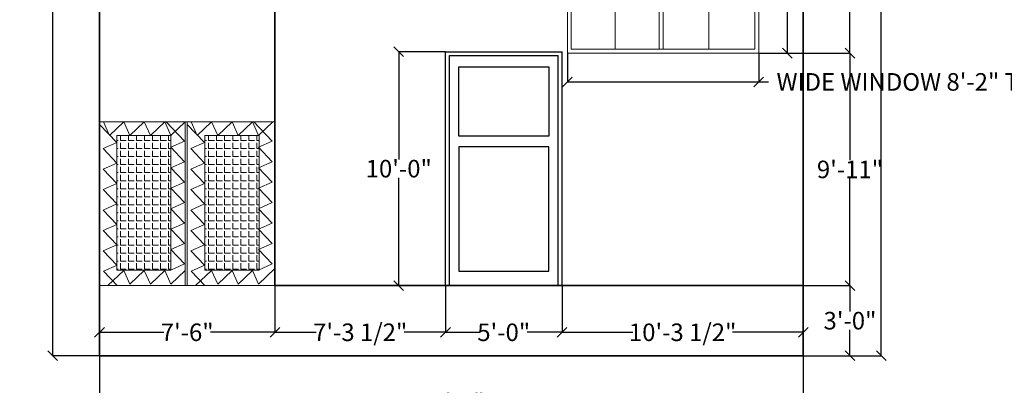
# Model space of a CAD drawing. Units: inches. Extents: x -19 to 1000, y -122 to 1144.
# Tile 6 of 8: x -19 to 486, y 313 to 501. Entities that reach past the tile are written whole.
import ezdxf

# ---------------------------------------------------------------- set-up
doc = ezdxf.new("R2010")
doc.units = ezdxf.units.IN
doc.header["$MEASUREMENT"] = 0
for name, color, linetype, lineweight in [('A-ANNO-DIMS', 191, 'Continuous', 18), ('A-ELEV', 4, 'Continuous', 35), ('A-ELEV-DOOR', 2, 'Continuous', 25), ('A-ELEV-GATE', 4, 'Continuous', 18), ('A-ELEV-GLAZ', 3, 'Continuous', 18), ('A-ELEV-PATT', 8, 'Continuous', 13)]:
    doc.layers.add(name, color=color, linetype=linetype, lineweight=lineweight)
doc.styles.get("Standard").update_dxf_attribs({"font": 'arial.ttf'})
doc.dimstyles.get("Standard").update_dxf_attribs({"dimtxt": 9, "dimasz": 5, "dimexe": 0.18, "dimexo": 0.0625, "dimgap": 0.09, "dimtad": 0, "dimtih": 1, "dimtoh": 1, "dimdec": 0, "dimzin": 0, "dimdsep": 46, "dimlunit": 3, "dimtxsty": 'Standard', "dimblk": 'OBLIQUE', "dimcen": 0.09, "dimadec": 0, "dimazin": 0, "dimtfac": 1, "dimtdec": 0, "dimtofl": 0, "dimtmove": 0, "dimatfit": 3, "dimfxl": 1, "dimtolj": 1, "dimtzin": 0, "dimarcsym": 0})

# ---------------------------------------------------------------- blocks, each defined once
blk = doc.blocks.new('_Oblique')
at = {"color": 0, "linetype": 'ByBlock', "lineweight": -2}
blk.add_line((-0.5, -0.5), (0.5, 0.5), dxfattribs=at)
blk = doc.blocks.new('*D9')
at = {"layer": 'A-ANNO-DIMS', "color": 0, "lineweight": -2, "transparency": 16777216}
for p, q in [((382.7, 727.13), (422.85, 727.13)), ((422.67, 727.13), (422.67, 532.32)), ((422.67, 328.13), (422.67, 522.95)), ((382.7, 328.13), (422.85, 328.13))]:
    blk.add_line(p, q, dxfattribs=at)
at = {"layer": 'Defpoints', "color": 0, "transparency": 16777216}
for p in [(382.64, 727.13), (422.67, 727.13), (382.64, 328.13)]:
    blk.add_point(p, dxfattribs=at)
at = {"layer": 'A-ANNO-DIMS', "color": 0, "lineweight": -2, "transparency": 16777216, "xscale": 5, "yscale": 5, "zscale": 5}
for p, rotation in [((422.67, 727.13), 90), ((422.67, 328.13), 270)]:
    blk.add_blockref('_Oblique', p, dxfattribs=dict(at, rotation=rotation))
at = {"layer": 'A-ANNO-DIMS', "color": 0, "transparency": 16777216, "insert": (422.67, 527.63), "char_height": 9, "attachment_point": 5}
blk.add_mtext('\\A1;33\'-3"', dxfattribs=at)
blk = doc.blocks.new('WINDOW-ELEV-WIDE')
for p, q in [((47.06, 49.36), (47.06, 64.32)), ((49.06, 49.36), (49.06, 64.32)), ((2, 49.36), (47.06, 49.36)), ((2, 47.36), (47.06, 47.36)), ((24.53, 47.36), (24.53, 2)), ((47.06, 2), (47.06, 47.36)), ((49.06, 49.36), (96.11, 49.36)), ((49.06, 2), (49.06, 47.36)), ((49.06, 47.36), (96.11, 47.36)), ((72.58, 47.36), (72.58, 2))]:
    blk.add_line(p, q)
for points in [[(98.11, 0), (0, 0), (0, 66.32), (98.11, 66.32)], [(96.11, 2), (2, 2), (2, 64.32), (96.11, 64.32)]]:
    blk.add_lwpolyline(points, close=True)
blk = doc.blocks.new('*D73')
at = {"layer": 'A-ANNO-DIMS', "color": 0, "lineweight": -2, "transparency": 16777216}
for p, q in [((261.67, 483.28), (261.67, 468.45)), ((359.78, 483.28), (359.78, 468.45)), ((261.67, 468.63), (359.78, 468.63)), ((359.78, 468.63), (364.78, 468.63))]:
    blk.add_line(p, q, dxfattribs=at)
at = {"layer": 'Defpoints', "color": 0, "transparency": 16777216}
for p in [(261.67, 483.35), (359.78, 483.35), (359.78, 468.63)]:
    blk.add_point(p, dxfattribs=at)
at = {"layer": 'A-ANNO-DIMS', "color": 0, "lineweight": -2, "transparency": 16777216, "xscale": 5, "yscale": 5, "zscale": 5, "rotation": 180}
blk.add_blockref('_Oblique', (261.67, 468.63), dxfattribs=at)
at = {"layer": 'A-ANNO-DIMS', "color": 0, "lineweight": -2, "transparency": 16777216, "xscale": 5, "yscale": 5, "zscale": 5}
blk.add_blockref('_Oblique', (359.78, 468.63), dxfattribs=at)
at = {"layer": 'A-ANNO-DIMS', "color": 0, "transparency": 16777216, "insert": (439.97, 468.63), "char_height": 9, "attachment_point": 5}
blk.add_mtext('\\A1;WIDE WINDOW 8\'-2" TYP.', dxfattribs=at)
blk = doc.blocks.new('*D74')
at = {"layer": 'A-ANNO-DIMS', "color": 0, "lineweight": -2, "transparency": 16777216}
for p, q in [((359.84, 549.66), (374.68, 549.66)), ((374.5, 549.66), (374.5, 521.25)), ((374.5, 483.35), (374.5, 511.76)), ((359.84, 483.35), (374.68, 483.35))]:
    blk.add_line(p, q, dxfattribs=at)
at = {"layer": 'Defpoints', "color": 0, "transparency": 16777216}
for p in [(359.78, 549.66), (374.5, 549.66), (359.78, 483.35)]:
    blk.add_point(p, dxfattribs=at)
at = {"layer": 'A-ANNO-DIMS', "color": 0, "lineweight": -2, "transparency": 16777216, "xscale": 5, "yscale": 5, "zscale": 5}
for p, rotation in [((374.5, 549.66), 90), ((374.5, 483.35), 270)]:
    blk.add_blockref('_Oblique', p, dxfattribs=dict(at, rotation=rotation))
at = {"layer": 'A-ANNO-DIMS', "color": 0, "transparency": 16777216, "insert": (374.5, 516.51), "char_height": 9, "attachment_point": 5}
blk.add_mtext('\\A1;5\'-6 1/2" TYP.', dxfattribs=at)
blk = doc.blocks.new('*D78')
at = {"layer": 'A-ANNO-DIMS', "color": 0, "lineweight": -2, "transparency": 16777216}
for p, q in [((61.2, 524.21), (61.2, 509.56)), ((83.4, 524.21), (83.4, 509.56)), ((61.2, 509.74), (83.4, 509.74)), ((83.4, 509.74), (88.4, 509.74))]:
    blk.add_line(p, q, dxfattribs=at)
at = {"layer": 'Defpoints', "color": 0, "transparency": 16777216}
for p in [(61.2, 524.27), (83.4, 524.27), (83.4, 509.74)]:
    blk.add_point(p, dxfattribs=at)
at = {"layer": 'A-ANNO-DIMS', "color": 0, "lineweight": -2, "transparency": 16777216, "xscale": 5, "yscale": 5, "zscale": 5, "rotation": 180}
blk.add_blockref('_Oblique', (61.2, 509.74), dxfattribs=at)
at = {"layer": 'A-ANNO-DIMS', "color": 0, "lineweight": -2, "transparency": 16777216, "xscale": 5, "yscale": 5, "zscale": 5}
blk.add_blockref('_Oblique', (83.4, 509.74), dxfattribs=at)
at = {"layer": 'A-ANNO-DIMS', "color": 0, "transparency": 16777216, "insert": (118.99, 509.74), "char_height": 9, "attachment_point": 5}
blk.add_mtext('\\A1;1\'-10" TYP.', dxfattribs=at)
blk = doc.blocks.new('*D111')
at = {"layer": 'A-ANNO-DIMS', "color": 0, "lineweight": -2, "transparency": 16777216}
for p, q in [((21.64, 328.07), (21.64, 304)), ((382.64, 328.07), (382.64, 304)), ((21.64, 304.18), (186.6, 304.18)), ((382.64, 304.18), (217.69, 304.18))]:
    blk.add_line(p, q, dxfattribs=at)
at = {"layer": 'Defpoints', "color": 0, "transparency": 16777216}
for p in [(21.64, 328.13), (382.64, 328.13), (21.64, 304.18)]:
    blk.add_point(p, dxfattribs=at)
at = {"layer": 'A-ANNO-DIMS', "color": 0, "lineweight": -2, "transparency": 16777216, "xscale": 5, "yscale": 5, "zscale": 5, "rotation": 180}
blk.add_blockref('_Oblique', (21.64, 304.18), dxfattribs=at)
at = {"layer": 'A-ANNO-DIMS', "color": 0, "lineweight": -2, "transparency": 16777216, "xscale": 5, "yscale": 5, "zscale": 5}
blk.add_blockref('_Oblique', (382.64, 304.18), dxfattribs=at)
at = {"layer": 'A-ANNO-DIMS', "color": 0, "transparency": 16777216, "insert": (202.14, 304.18), "char_height": 9, "attachment_point": 5}
blk.add_mtext('\\A1;30\'-1"', dxfattribs=at)
blk = doc.blocks.new('*D112')
at = {"layer": 'A-ANNO-DIMS', "color": 0, "lineweight": -2, "transparency": 16777216}
for p, q in [((21.58, 797.3), (-2.49, 797.3)), ((-2.31, 797.3), (-2.31, 567.4)), ((-2.31, 328.13), (-2.31, 558.03)), ((21.58, 328.13), (-2.49, 328.13))]:
    blk.add_line(p, q, dxfattribs=at)
at = {"layer": 'Defpoints', "color": 0, "transparency": 16777216}
for p in [(-2.31, 797.3), (21.64, 797.3), (21.64, 328.13)]:
    blk.add_point(p, dxfattribs=at)
at = {"layer": 'A-ANNO-DIMS', "color": 0, "lineweight": -2, "transparency": 16777216, "xscale": 5, "yscale": 5, "zscale": 5}
for p, rotation in [((-2.31, 797.3), 90), ((-2.31, 328.13), 270)]:
    blk.add_blockref('_Oblique', p, dxfattribs=dict(at, rotation=rotation))
at = {"layer": 'A-ANNO-DIMS', "color": 0, "transparency": 16777216, "insert": (-2.31, 562.72), "char_height": 9, "attachment_point": 5}
blk.add_mtext('\\A1;39\'-1"', dxfattribs=at)
blk = doc.blocks.new('*D113')
at = {"layer": 'A-ANNO-DIMS', "color": 0, "lineweight": -2, "transparency": 16777216}
for p, q in [((21.64, 364.07), (21.64, 340)), ((111.64, 364.07), (111.64, 340)), ((21.64, 340.18), (54.63, 340.18)), ((111.64, 340.18), (78.66, 340.18))]:
    blk.add_line(p, q, dxfattribs=at)
at = {"layer": 'Defpoints', "color": 0, "transparency": 16777216}
for p in [(21.64, 364.13), (111.64, 364.13), (21.64, 340.18)]:
    blk.add_point(p, dxfattribs=at)
at = {"layer": 'A-ANNO-DIMS', "color": 0, "lineweight": -2, "transparency": 16777216, "xscale": 5, "yscale": 5, "zscale": 5, "rotation": 180}
blk.add_blockref('_Oblique', (21.64, 340.18), dxfattribs=at)
at = {"layer": 'A-ANNO-DIMS', "color": 0, "lineweight": -2, "transparency": 16777216, "xscale": 5, "yscale": 5, "zscale": 5}
blk.add_blockref('_Oblique', (111.64, 340.18), dxfattribs=at)
at = {"layer": 'A-ANNO-DIMS', "color": 0, "transparency": 16777216, "insert": (66.64, 340.18), "char_height": 9, "attachment_point": 5}
blk.add_mtext('\\A1;7\'-6"', dxfattribs=at)
blk = doc.blocks.new('*D114')
at = {"layer": 'A-ANNO-DIMS', "color": 0, "lineweight": -2, "transparency": 16777216}
for p, q in [((111.64, 364.07), (111.64, 340)), ((199.11, 364.07), (199.11, 340)), ((111.64, 340.18), (132.87, 340.18)), ((199.11, 340.18), (177.88, 340.18))]:
    blk.add_line(p, q, dxfattribs=at)
at = {"layer": 'Defpoints', "color": 0, "transparency": 16777216}
for p in [(111.64, 364.13), (199.11, 364.13), (111.64, 340.18)]:
    blk.add_point(p, dxfattribs=at)
at = {"layer": 'A-ANNO-DIMS', "color": 0, "lineweight": -2, "transparency": 16777216, "xscale": 5, "yscale": 5, "zscale": 5, "rotation": 180.0000000000001}
blk.add_blockref('_Oblique', (111.64, 340.18), dxfattribs=at)
at = {"layer": 'A-ANNO-DIMS', "color": 0, "lineweight": -2, "transparency": 16777216, "xscale": 5, "yscale": 5, "zscale": 5}
blk.add_blockref('_Oblique', (199.11, 340.18), dxfattribs=at)
at = {"layer": 'A-ANNO-DIMS', "color": 0, "transparency": 16777216, "insert": (155.38, 340.18), "char_height": 9, "attachment_point": 5}
blk.add_mtext('\\A1;7\'-3 1/2"', dxfattribs=at)
blk = doc.blocks.new('*D115')
at = {"layer": 'A-ANNO-DIMS', "color": 0, "lineweight": -2, "transparency": 16777216}
for p, q in [((199.11, 364.07), (199.11, 340)), ((258.9, 364.07), (258.9, 340)), ((199.11, 340.18), (216.95, 340.18)), ((258.9, 340.18), (241.06, 340.18))]:
    blk.add_line(p, q, dxfattribs=at)
at = {"layer": 'Defpoints', "color": 0, "transparency": 16777216}
for p in [(199.11, 364.13), (258.9, 364.13), (199.11, 340.18)]:
    blk.add_point(p, dxfattribs=at)
at = {"layer": 'A-ANNO-DIMS', "color": 0, "lineweight": -2, "transparency": 16777216, "xscale": 5, "yscale": 5, "zscale": 5, "rotation": 180}
blk.add_blockref('_Oblique', (199.11, 340.18), dxfattribs=at)
at = {"layer": 'A-ANNO-DIMS', "color": 0, "lineweight": -2, "transparency": 16777216, "xscale": 5, "yscale": 5, "zscale": 5}
blk.add_blockref('_Oblique', (258.9, 340.18), dxfattribs=at)
at = {"layer": 'A-ANNO-DIMS', "color": 0, "transparency": 16777216, "insert": (229, 340.18), "char_height": 9, "attachment_point": 5}
blk.add_mtext('\\A1;5\'-0"', dxfattribs=at)
blk = doc.blocks.new('*D116')
at = {"layer": 'A-ANNO-DIMS', "color": 0, "lineweight": -2, "transparency": 16777216}
for p, q in [((258.9, 364.07), (258.9, 340)), ((382.64, 364.07), (382.64, 340)), ((258.9, 340.18), (295.16, 340.18)), ((382.64, 340.18), (346.38, 340.18))]:
    blk.add_line(p, q, dxfattribs=at)
at = {"layer": 'Defpoints', "color": 0, "transparency": 16777216}
for p in [(258.9, 364.13), (382.64, 364.13), (258.9, 340.18)]:
    blk.add_point(p, dxfattribs=at)
at = {"layer": 'A-ANNO-DIMS', "color": 0, "lineweight": -2, "transparency": 16777216, "xscale": 5, "yscale": 5, "zscale": 5}
for p, rotation in [((258.9, 340.18), 179.9999999999999), ((382.64, 340.18), 359.9999999999999)]:
    blk.add_blockref('_Oblique', p, dxfattribs=dict(at, rotation=rotation))
at = {"layer": 'A-ANNO-DIMS', "color": 0, "transparency": 16777216, "insert": (320.77, 340.18), "char_height": 9, "attachment_point": 5}
blk.add_mtext('\\A1;10\'-3 1/2"', dxfattribs=at)
blk = doc.blocks.new('*D117')
at = {"layer": 'A-ANNO-DIMS', "color": 0, "lineweight": -2, "transparency": 16777216}
for p, q in [((382.7, 364.13), (406.77, 364.13)), ((406.59, 364.13), (406.59, 350.82)), ((406.59, 328.13), (406.59, 341.45)), ((382.7, 328.13), (406.77, 328.13))]:
    blk.add_line(p, q, dxfattribs=at)
at = {"layer": 'Defpoints', "color": 0, "transparency": 16777216}
for p in [(382.64, 364.13), (406.59, 364.13), (382.64, 328.13)]:
    blk.add_point(p, dxfattribs=at)
at = {"layer": 'A-ANNO-DIMS', "color": 0, "lineweight": -2, "transparency": 16777216, "xscale": 5, "yscale": 5, "zscale": 5}
for p, rotation in [((406.59, 364.13), 90), ((406.59, 328.13), 270)]:
    blk.add_blockref('_Oblique', p, dxfattribs=dict(at, rotation=rotation))
at = {"layer": 'A-ANNO-DIMS', "color": 0, "transparency": 16777216, "insert": (406.59, 346.13), "char_height": 9, "attachment_point": 5}
blk.add_mtext('\\A1;3\'-0"', dxfattribs=at)
blk = doc.blocks.new('*D118')
at = {"layer": 'A-ANNO-DIMS', "color": 0, "lineweight": -2, "transparency": 16777216}
for p, q in [((199.05, 484.13), (174.98, 484.13)), ((175.16, 484.13), (175.16, 428.82)), ((175.16, 364.13), (175.16, 419.45)), ((199.05, 364.13), (174.98, 364.13))]:
    blk.add_line(p, q, dxfattribs=at)
at = {"layer": 'Defpoints', "color": 0, "transparency": 16777216}
for p in [(175.16, 484.13), (199.11, 484.13), (199.11, 364.13)]:
    blk.add_point(p, dxfattribs=at)
at = {"layer": 'A-ANNO-DIMS', "color": 0, "lineweight": -2, "transparency": 16777216, "xscale": 5, "yscale": 5, "zscale": 5}
for p, rotation in [((175.16, 484.13), 90), ((175.16, 364.13), 270)]:
    blk.add_blockref('_Oblique', p, dxfattribs=dict(at, rotation=rotation))
at = {"layer": 'A-ANNO-DIMS', "color": 0, "transparency": 16777216, "insert": (175.16, 424.13), "char_height": 9, "attachment_point": 5}
blk.add_mtext('\\A1;10\'-0"', dxfattribs=at)
blk = doc.blocks.new('*D121')
at = {"layer": 'A-ANNO-DIMS', "color": 0, "lineweight": -2, "transparency": 16777216}
for p, q in [((359.84, 483.35), (406.77, 483.35)), ((406.59, 483.35), (406.59, 428.43)), ((406.59, 364.13), (406.59, 419.06)), ((382.7, 364.13), (406.77, 364.13))]:
    blk.add_line(p, q, dxfattribs=at)
at = {"layer": 'Defpoints', "color": 0, "transparency": 16777216}
for p in [(359.78, 483.35), (406.59, 483.35), (382.64, 364.13)]:
    blk.add_point(p, dxfattribs=at)
at = {"layer": 'A-ANNO-DIMS', "color": 0, "lineweight": -2, "transparency": 16777216, "xscale": 5, "yscale": 5, "zscale": 5}
for p, rotation in [((406.59, 483.35), 90), ((406.59, 364.13), 270)]:
    blk.add_blockref('_Oblique', p, dxfattribs=dict(at, rotation=rotation))
at = {"layer": 'A-ANNO-DIMS', "color": 0, "transparency": 16777216, "insert": (406.59, 423.74), "char_height": 9, "attachment_point": 5}
blk.add_mtext('\\A1;9\'-11"', dxfattribs=at)
blk = doc.blocks.new('*D122')
at = {"layer": 'A-ANNO-DIMS', "color": 0, "lineweight": -2, "transparency": 16777216}
for p, q in [((382.7, 613.85), (406.77, 613.85)), ((406.59, 613.85), (406.59, 553.34)), ((406.59, 483.35), (406.59, 543.86)), ((359.84, 483.35), (406.77, 483.35))]:
    blk.add_line(p, q, dxfattribs=at)
at = {"layer": 'Defpoints', "color": 0, "transparency": 16777216}
for p in [(382.64, 613.85), (406.59, 613.85), (359.78, 483.35)]:
    blk.add_point(p, dxfattribs=at)
at = {"layer": 'A-ANNO-DIMS', "color": 0, "lineweight": -2, "transparency": 16777216, "xscale": 5, "yscale": 5, "zscale": 5}
for p, rotation in [((406.59, 613.85), 90), ((406.59, 483.35), 270)]:
    blk.add_blockref('_Oblique', p, dxfattribs=dict(at, rotation=rotation))
at = {"layer": 'A-ANNO-DIMS', "color": 0, "transparency": 16777216, "insert": (406.59, 548.6), "char_height": 9, "attachment_point": 5}
blk.add_mtext('\\A1;10\'-10 1/2"', dxfattribs=at)

msp = doc.modelspace()

# ---------------------------------------------------------------- hatches: boundary and pattern name
at = {"layer": 'A-ELEV-PATT'}
h = msp.add_hatch(dxfattribs=at)
h.set_pattern_fill('ANGLE', color=256, scale=15)
h.set_pattern_definition([(0, (-437.899, -266.802), (0, 4.125), [3, -1.125]), (90, (-437.899, -266.802), (-4.125, 3e-16), [3, -1.125])])
h.paths.add_polyline_path([(58.27, 441.14), (30.51, 441.14), (30.51, 372.1), (58.27, 372.1)])
h = msp.add_hatch(dxfattribs=at)
h.set_pattern_fill('ANGLE', color=256, scale=15)
h.set_pattern_definition([(0, (-392.659, -266.802), (0, 4.125), [3, -1.125]), (90, (-392.659, -266.802), (-4.125, 3e-16), [3, -1.125])])
h.paths.add_polyline_path([(103.51, 441.14), (75.75, 441.14), (75.75, 372.1), (103.51, 372.1)])

# ---------------------------------------------------------------- linework, layer by layer
at = {"layer": 'A-ELEV'}
for p, q in [((21.64, 328.13), (21.64, 727.13)), ((111.64, 364.13), (111.64, 727.13)), ((382.64, 328.13), (382.64, 727.13)), ((382.64, 328.13), (382.64, 727.13)), ((382.64, 364.13), (111.64, 364.13)), ((382.64, 328.13), (21.64, 328.13))]:
    msp.add_line(p, q, dxfattribs=at)
at = {"layer": 'A-ELEV-DOOR'}
for p, q in [((199.11, 364.13), (199.11, 484.13)), ((199.11, 484.13), (258.9, 484.13)), ((201.11, 482.13), (256.9, 482.13)), ((201.11, 364.13), (201.11, 482.13)), ((256.9, 364.13), (256.9, 482.13)), ((258.9, 364.13), (258.9, 484.13))]:
    msp.add_line(p, q, dxfattribs=at)
for points in [[(252.13, 440.81), (206.02, 440.81), (206.02, 476.32), (252.13, 476.32)], [(252.13, 435.3), (206.02, 435.3), (206.02, 371.57), (252.13, 371.57)]]:
    msp.add_lwpolyline(points, close=True, dxfattribs=at)
at = {"layer": 'A-ELEV-GATE'}
for p, q in [((111.64, 448.13), (21.64, 448.13)), ((21.64, 446.86), (30.51, 437.5)), ((26.78, 441.14), (23.66, 448.13)), ((26.78, 441.14), (34.15, 448.13)), ((37.28, 441.14), (34.15, 448.13)), ((37.28, 441.14), (44.65, 448.13)), ((47.77, 441.14), (44.65, 448.13)), ((47.77, 441.14), (55.15, 448.13)), ((58.27, 441.14), (55.15, 448.13)), ((65.26, 438.2), (55.84, 448.13)), ((58.27, 441.14), (65.64, 448.13)), ((65.64, 364.13), (65.64, 448.13)), ((66.64, 364.13), (66.64, 448.13)), ((66.64, 446.86), (75.51, 437.5)), ((71.78, 441.14), (68.66, 448.13)), ((71.78, 441.14), (79.15, 448.13)), ((82.28, 441.14), (79.15, 448.13)), ((82.28, 441.14), (89.65, 448.13)), ((92.77, 441.14), (89.65, 448.13)), ((92.77, 441.14), (100.15, 448.13)), ((103.27, 441.14), (100.15, 448.13)), ((110.26, 438.2), (100.84, 448.13)), ((103.27, 441.14), (110.64, 448.13)), ((23.53, 434.38), (30.51, 437.5)), ((23.53, 434.38), (30.51, 427.01)), ((65.26, 438.2), (58.27, 435.08)), ((65.26, 427.7), (58.27, 435.08)), ((68.53, 434.38), (75.51, 437.5)), ((68.53, 434.38), (75.51, 427.01)), ((110.26, 438.2), (103.27, 435.08)), ((110.26, 427.7), (103.27, 435.08)), ((23.53, 423.88), (30.51, 427.01)), ((65.26, 427.7), (58.27, 424.58)), ((65.26, 417.21), (58.27, 424.58)), ((68.53, 423.88), (75.51, 427.01)), ((110.26, 427.7), (103.27, 424.58)), ((110.26, 417.21), (103.27, 424.58)), ((23.53, 423.88), (30.51, 416.51)), ((68.53, 423.88), (75.51, 416.51)), ((23.53, 413.39), (30.51, 416.51)), ((65.26, 417.21), (58.27, 414.08)), ((68.53, 413.39), (75.51, 416.51)), ((110.26, 417.21), (103.27, 414.08)), ((23.53, 413.39), (30.51, 406.01)), ((65.26, 406.71), (58.27, 414.08)), ((68.53, 413.39), (75.51, 406.01)), ((110.26, 406.71), (103.27, 414.08)), ((23.53, 402.89), (30.51, 406.01)), ((65.26, 406.71), (58.27, 403.59)), ((68.53, 402.89), (75.51, 406.01)), ((110.26, 406.71), (103.27, 403.59)), ((23.53, 402.89), (30.51, 395.52)), ((65.26, 396.21), (58.27, 403.59)), ((68.53, 402.89), (75.51, 395.52)), ((110.26, 396.21), (103.27, 403.59)), ((23.53, 392.39), (30.51, 395.52)), ((65.26, 396.21), (58.27, 393.09)), ((68.53, 392.39), (75.51, 395.52)), ((110.26, 396.21), (103.27, 393.09)), ((23.53, 392.39), (30.51, 385.02)), ((65.26, 385.72), (58.27, 393.09)), ((68.53, 392.39), (75.51, 385.02)), ((110.26, 385.72), (103.27, 393.09)), ((23.53, 381.9), (30.51, 385.02)), ((65.26, 385.72), (58.27, 382.6)), ((68.53, 381.9), (75.51, 385.02)), ((110.26, 385.72), (103.27, 382.6)), ((23.53, 381.9), (30.51, 374.53)), ((65.26, 375.22), (58.27, 382.6)), ((68.53, 381.9), (75.51, 374.53)), ((110.26, 375.22), (103.27, 382.6)), ((23.76, 371.51), (30.75, 374.63)), ((65.26, 375.22), (58.27, 372.1)), ((68.76, 371.51), (75.75, 374.63)), ((110.26, 375.22), (103.27, 372.1)), ((23.76, 371.51), (30.75, 364.13)), ((25.94, 364.13), (34.15, 371.92)), ((37.28, 364.93), (34.15, 371.92)), ((37.28, 364.93), (44.65, 371.92)), ((47.77, 364.93), (44.65, 371.92)), ((47.77, 364.93), (55.15, 371.92)), ((58.27, 364.93), (55.15, 371.92)), ((58.27, 364.93), (65.64, 371.92)), ((68.76, 371.51), (75.75, 364.13)), ((70.94, 364.13), (79.15, 371.92)), ((82.28, 364.93), (79.15, 371.92)), ((82.28, 364.93), (89.65, 371.92)), ((92.77, 364.93), (89.65, 371.92)), ((92.77, 364.93), (100.15, 371.92)), ((103.27, 364.93), (100.15, 371.92)), ((103.27, 364.93), (111.64, 372.87)), ((111.64, 364.13), (21.64, 364.13))]:
    msp.add_line(p, q, dxfattribs=at)
for points in [[(58.27, 372.1), (30.51, 372.1), (30.51, 441.14), (58.27, 441.14)], [(103.51, 372.1), (75.75, 372.1), (75.75, 441.14), (103.51, 441.14)]]:
    msp.add_lwpolyline(points, close=True, dxfattribs=at)

# ---------------------------------------------------------------- block references
at = {"layer": 'A-ELEV-GLAZ'}
msp.add_blockref('WINDOW-ELEV-WIDE', (261.67, 483.35), dxfattribs=at)

# ---------------------------------------------------------------- dimensions: what is measured, and where the dimension line sits
at = {"layer": 'A-ANNO-DIMS'}
for base, p1, p2, angle, override, picture, middle in [((-2.31, 797.3), (21.64, 328.13), (21.64, 797.3), 90, {"dimdec": 1, "dimlfac": 1, "dimrnd": 0, "dimzin": 1, "dimdsep": 46, "dimlunit": 4, "dimfrac": 2}, '*D112', (-2.31, 562.72)), ((422.67, 727.13), (382.64, 328.13), (382.64, 727.13), 90, {"dimclrd": 0, "dimclre": 0, "dimclrt": 0}, '*D9', (422.67, 527.63)), ((406.59, 613.85), (359.78, 483.35), (382.64, 613.85), 90, {"dimdec": 1, "dimlfac": 1, "dimrnd": 0, "dimzin": 1, "dimdsep": 46, "dimlunit": 4, "dimfrac": 2}, '*D122', (406.59, 548.6)), ((175.16, 484.13), (199.11, 364.13), (199.11, 484.13), 90, {"dimdec": 1, "dimlfac": 1, "dimrnd": 0, "dimzin": 1, "dimdsep": 46, "dimlunit": 4, "dimfrac": 2}, '*D118', (175.16, 424.13)), ((406.59, 483.35), (382.64, 364.13), (359.78, 483.35), 90, {"dimdec": 1, "dimlfac": 1, "dimrnd": 0, "dimzin": 1, "dimdsep": 46, "dimlunit": 4, "dimfrac": 2}, '*D121', (406.59, 423.74)), ((21.64, 340.18), (111.64, 364.13), (21.64, 364.13), 180, {"dimdec": 1, "dimlfac": 1, "dimrnd": 0, "dimzin": 1, "dimdsep": 46, "dimlunit": 4, "dimfrac": 2}, '*D113', (66.64, 340.18)), ((111.64, 340.18), (199.11, 364.13), (111.64, 364.13), 180, {"dimdec": 1, "dimlfac": 1, "dimrnd": 0, "dimzin": 1, "dimdsep": 46, "dimlunit": 4, "dimfrac": 2}, '*D114', (155.38, 340.18)), ((199.11, 340.18), (258.9, 364.13), (199.11, 364.13), 180, {"dimdec": 1, "dimlfac": 1, "dimrnd": 0, "dimzin": 1, "dimdsep": 46, "dimlunit": 4, "dimfrac": 2}, '*D115', (229, 340.18)), ((258.9, 340.18), (382.64, 364.13), (258.9, 364.13), 180, {"dimdec": 1, "dimlfac": 1, "dimrnd": 0, "dimzin": 1, "dimdsep": 46, "dimlunit": 4, "dimfrac": 2}, '*D116', (320.77, 340.18)), ((406.59, 364.13), (382.64, 328.13), (382.64, 364.13), 90, {"dimdec": 1, "dimlfac": 1, "dimrnd": 0, "dimzin": 1, "dimdsep": 46, "dimlunit": 4, "dimfrac": 2}, '*D117', (406.59, 346.13)), ((21.64, 304.18), (382.64, 328.13), (21.64, 328.13), 180, {"dimdec": 1, "dimlfac": 1, "dimrnd": 0, "dimzin": 1, "dimdsep": 46, "dimlunit": 4, "dimfrac": 2}, '*D111', (202.14, 304.18))]:
    dim = msp.add_linear_dim(base=base, p1=p1, p2=p2, angle=angle, dimstyle='Standard', override=override, dxfattribs=at)
    dim.commit()
    dim.dimension.update_dxf_attribs({"geometry": picture, "text_midpoint": middle})
dim = msp.add_linear_dim(base=(374.5, 549.66), p1=(359.78, 483.35), p2=(359.78, 549.66), angle=90, text='<> TYP.', dimstyle='Standard', override={"dimdec": 1, "dimlfac": 1, "dimrnd": 0, "dimzin": 1, "dimdsep": 46, "dimlunit": 4, "dimfrac": 2}, dxfattribs=at)
dim.commit()
dim.dimension.update_dxf_attribs({"geometry": '*D74', "text_midpoint": (374.5, 516.51)})
for base, p1, p2, text, picture, middle in [((83.4, 509.74), (61.2, 524.27), (83.4, 524.27), '<> TYP.', '*D78', (118.99, 509.74)), ((359.78, 468.63), (261.67, 483.35), (359.78, 483.35), 'WIDE WINDOW <> TYP.', '*D73', (439.97, 468.63))]:
    dim = msp.add_linear_dim(base=base, p1=p1, p2=p2, text=text, dimstyle='Standard', override={"dimdec": 1, "dimlfac": 1, "dimrnd": 0, "dimzin": 1, "dimdsep": 46, "dimlunit": 4, "dimfrac": 2}, dxfattribs=at)
    dim.commit()
    dim.dimension.update_dxf_attribs({"geometry": picture, "text_midpoint": middle})

doc.saveas('drawing.dxf')
